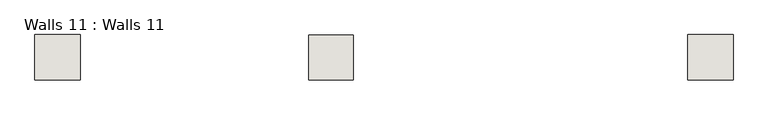
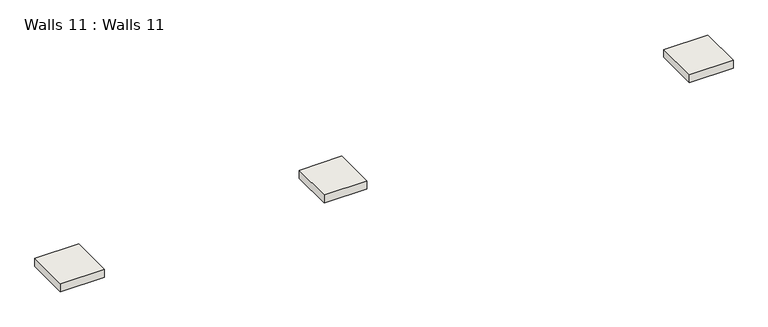
"""IFC4 building model written with IfcOpenShell, lengths in millimetres: wall geometry, Walls 11 : Walls 11."""

from ifc_helpers import new_model, si_unit, frame, origin, place, context, project, spatial, polyline, outline, extrude, source, transform, mapped, element, save


def walls_11_walls_11_b291a2b5(model_context):
    return source(origin(), model_context, "Body", "SweptSolid", [
        extrude(outline(polyline([(-4643.9305193, -4666.7213241), (-5202.7305193, -4666.7213241), (-5202.7305193, -4107.9213241), (-4643.9305193, -4107.9213241), (-4643.9305193, -4666.7213241)])), frame((0.0, 0.0, 2117.227688), z_axis=(0.0, 0.0, 1.0), x_axis=(1.0, 0.0, 0.0)), (0.0, 0.0, 1.0), 108.9204974),
        extrude(outline(polyline([(3379.0074298, -4666.7213241), (2820.2074298, -4666.7213241), (2820.2074298, -4107.9213241), (3379.0074298, -4107.9213241), (3379.0074298, -4666.7213241)])), frame((0.0, 0.0, 2133.6), z_axis=(0.0, 0.0, 1.0), x_axis=(1.0, 0.0, 0.0)), (0.0, 0.0, 1.0), 106.1422557),
        extrude(outline(polyline([(-1290.6968693, -4664.3450456), (-1836.7968693, -4664.3450456), (-1836.7968693, -4111.8950456), (-1290.6968693, -4111.8950456), (-1290.6968693, -4664.3450456)])), frame((0.0, 0.0, 2133.6), z_axis=(0.0, 0.0, 1.0), x_axis=(1.0, 0.0, 0.0)), (0.0, 0.0, 1.0), 108.2510602),
    ])


if __name__ == "__main__":
    model = new_model("IFC4")
    model_context = context("Model", 3, world=origin())
    ifc_project = project(units=[si_unit("LENGTHUNIT", "METRE", prefix="MILLI")], contexts=[model_context])
    site = spatial("IfcSite", under=ifc_project)
    building = spatial("IfcBuilding", under=site)
    placement = place(None, origin())
    walls_11_walls_11_shape = walls_11_walls_11_b291a2b5(model_context)
    element("IfcWall", 1, ObjectType="Walls 11 : Walls 11", at=placement, inside=building, context=model_context, shape_type="MappedRepresentation", body=[
        mapped(walls_11_walls_11_shape, transform((0.0, 0.0, 0.0), x_axis=(1.0, 0.0, 0.0), y_axis=(0.0, 1.0, 0.0), z_axis=(0.0, 0.0, 1.0))),
    ])
    save(model, "model.ifc")

# Revit data of these elements
# Element 1 (IfcWall, "Walls 11 : Walls 11")
#   Materials on its faces: "Default Wall"
# Materials
#   "Default Wall": colour RGB 128 128 128, transparency 0
